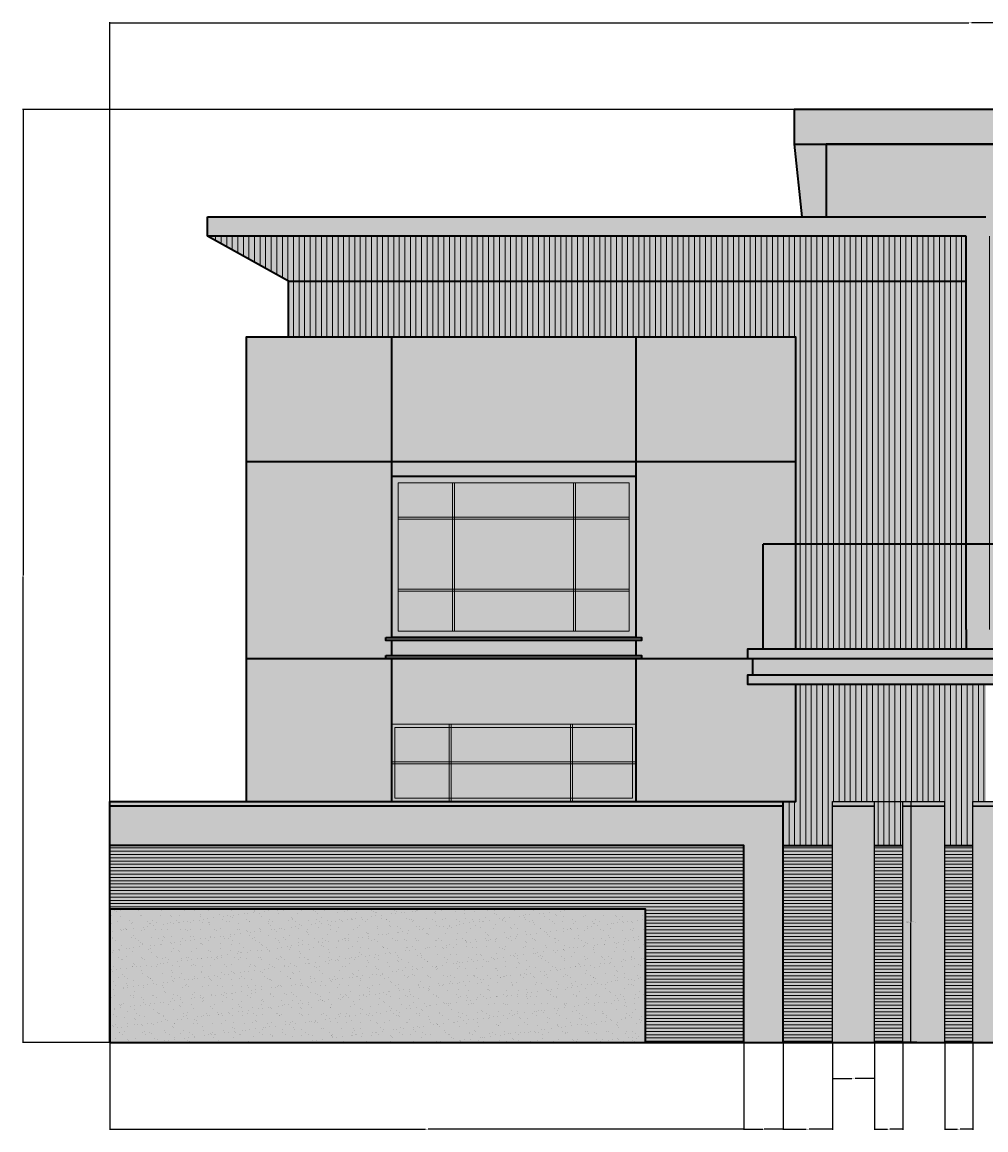
# Model space of a CAD drawing. Units: feet. Extents: x 2651 to 4047, y 949 to 1287.
# Tile 1 of 5: x 2651 to 2945, y 949 to 1287. Entities that reach past the tile are written whole.
import ezdxf

# ---------------------------------------------------------------- set-up
doc = ezdxf.new("R2010")
doc.units = ezdxf.units.FT
for name, color, linetype, lineweight in [('A-ANNO-DIMS', 2, 'Continuous', 18), ('A-ELEV', 7, 'Continuous', 35), ('A-ELEV-FNCE', 7, 'Continuous', 25), ('A-ELEV-PATT', 8, 'Continuous', 13), ('A-GLAZ', 4, 'Continuous', 18)]:
    doc.layers.add(name, color=color, linetype=linetype, lineweight=lineweight)
doc.styles.get("Standard").update_dxf_attribs({"font": 'arial.ttf'})
doc.dimstyles.get("Standard").update_dxf_attribs({"dimtxt": 0.18, "dimasz": 0.18, "dimexe": 0.18, "dimexo": 0.0625, "dimgap": 0.09, "dimtad": 0, "dimtih": 1, "dimtoh": 1, "dimdec": 1, "dimzin": 0, "dimdsep": 46, "dimlunit": 3, "dimtxsty": 'Standard', "dimcen": 0.09, "dimadec": 0, "dimazin": 0, "dimtfac": 1, "dimtdec": 1, "dimtofl": 0, "dimtmove": 0, "dimatfit": 3, "dimfxl": 1, "dimtolj": 1, "dimtzin": 0, "dimarcsym": 0})

# ---------------------------------------------------------------- blocks, each defined once
blk = doc.blocks.new('BOUNDARY-PIER-HATCHED')
for p, q in [((0, 72.1), (0, 73.54)), ((0, 72.1), (0, 73.54)), ((12.86, 0), (12.86, 73.54)), ((12.86, 0), (12.86, 73.54))]:
    blk.add_line(p, q)
for points in [[(0, 73.54), (12.86, 73.54)], [(0, 73.54), (12.86, 73.54)], [(12.86, 72.1), (0, 72.1)], [(12.86, 0), (0, 0), (0, 72.1), (12.86, 72.1)], [(12.86, 0), (0, 0), (0, 72.1), (12.86, 72.1)], [(12.86, 72.1), (0, 72.1)]]:
    blk.add_lwpolyline(points)
blk = doc.blocks.new('*D3')
at = {"layer": 'A-ANNO-DIMS', "color": 0, "lineweight": -2, "transparency": 16777216}
for p, q in [((2911.09, 1049.19), (2922.24, 1049.19)), ((2922.06, 1049.01), (2922.06, 1012.6)), ((2922.06, 975.83), (2922.06, 1012.23)), ((2911.09, 975.65), (2922.24, 975.65))]:
    blk.add_line(p, q, dxfattribs=at)
at = {"layer": 'A-ANNO-DIMS', "color": 0, "transparency": 16777216}
for points in [[(2922.03, 1049.01), (2922.09, 1049.01), (2922.06, 1049.19)], [(2922.03, 975.83), (2922.09, 975.83), (2922.06, 975.65)]]:
    blk.add_solid(points, dxfattribs=at)
at = {"layer": 'Defpoints', "color": 0, "transparency": 16777216}
for p in [(2911.03, 1049.19), (2922.06, 1049.19), (2911.03, 975.65)]:
    blk.add_point(p, dxfattribs=at)
at = {"layer": 'A-ANNO-DIMS', "color": 0, "transparency": 16777216, "insert": (2922.06, 1012.42), "char_height": 0.18, "attachment_point": 5}
blk.add_mtext('\\A1;BOUNDARY PIER 74 TYP.', dxfattribs=at)
blk = doc.blocks.new('*D4')
at = {"layer": 'A-ANNO-DIMS', "color": 0, "lineweight": -2, "transparency": 16777216}
for p, q in [((2898.17, 975.59), (2898.17, 964.44)), ((2911.03, 975.59), (2911.03, 964.44)), ((2898.35, 964.62), (2904.08, 964.62)), ((2910.85, 964.62), (2905.12, 964.62))]:
    blk.add_line(p, q, dxfattribs=at)
at = {"layer": 'A-ANNO-DIMS', "color": 0, "transparency": 16777216}
for points in [[(2898.35, 964.65), (2898.35, 964.59), (2898.17, 964.62)], [(2910.85, 964.65), (2910.85, 964.59), (2911.03, 964.62)]]:
    blk.add_solid(points, dxfattribs=at)
at = {"layer": 'Defpoints', "color": 0, "transparency": 16777216}
for p in [(2898.17, 975.65), (2911.03, 975.65), (2911.03, 964.62)]:
    blk.add_point(p, dxfattribs=at)
at = {"layer": 'A-ANNO-DIMS', "color": 0, "transparency": 16777216, "insert": (2904.6, 964.62), "char_height": 0.18, "attachment_point": 5}
blk.add_mtext('\\A1;13 TYP.', dxfattribs=at)
blk = doc.blocks.new('*D7')
at = {"layer": 'A-ANNO-DIMS', "color": 0, "lineweight": -2, "transparency": 16777216}
for p, q in [((2677.56, 975.71), (2677.56, 1287.01)), ((2677.74, 1286.83), (2939.77, 1286.83)), ((3202.59, 1286.83), (2940.56, 1286.83)), ((3202.77, 1095.71), (3202.77, 1287.01))]:
    blk.add_line(p, q, dxfattribs=at)
at = {"layer": 'A-ANNO-DIMS', "color": 0, "transparency": 16777216}
for points in [[(2677.74, 1286.86), (2677.74, 1286.8), (2677.56, 1286.83)], [(3202.59, 1286.86), (3202.59, 1286.8), (3202.77, 1286.83)]]:
    blk.add_solid(points, dxfattribs=at)
at = {"layer": 'Defpoints', "color": 0, "transparency": 16777216}
for p in [(3202.77, 1286.83), (3202.77, 1095.65), (2677.56, 975.65)]:
    blk.add_point(p, dxfattribs=at)
at = {"layer": 'A-ANNO-DIMS', "color": 0, "transparency": 16777216, "insert": (2940.17, 1286.83), "char_height": 0.18, "attachment_point": 5}
blk.add_mtext('\\A1;525.2', dxfattribs=at)
blk = doc.blocks.new('*D8')
at = {"layer": 'A-ANNO-DIMS', "color": 0, "lineweight": -2, "transparency": 16777216}
for p, q in [((3098.48, 1260.33), (2650.88, 1260.33)), ((2651.06, 1260.15), (2651.06, 1118.17)), ((2651.06, 975.83), (2651.06, 1117.81)), ((2677.49, 975.65), (2650.88, 975.65))]:
    blk.add_line(p, q, dxfattribs=at)
at = {"layer": 'A-ANNO-DIMS', "color": 0, "transparency": 16777216}
for points in [[(2651.03, 1260.15), (2651.09, 1260.15), (2651.06, 1260.33)], [(2651.03, 975.83), (2651.09, 975.83), (2651.06, 975.65)]]:
    blk.add_solid(points, dxfattribs=at)
at = {"layer": 'Defpoints', "color": 0, "transparency": 16777216}
for p in [(2651.06, 1260.33), (3098.55, 1260.33), (2677.56, 975.65)]:
    blk.add_point(p, dxfattribs=at)
at = {"layer": 'A-ANNO-DIMS', "color": 0, "transparency": 16777216, "insert": (2651.06, 1117.99), "char_height": 0.18, "attachment_point": 5}
blk.add_mtext('\\A1;284.7', dxfattribs=at)
blk = doc.blocks.new('*D9')
at = {"layer": 'A-ANNO-DIMS', "color": 0, "lineweight": -2, "transparency": 16777216}
for p, q in [((2677.56, 975.59), (2677.56, 948.97)), ((2871.06, 975.59), (2871.06, 948.97)), ((2677.74, 949.15), (2773.92, 949.15)), ((2870.88, 949.15), (2774.7, 949.15))]:
    blk.add_line(p, q, dxfattribs=at)
at = {"layer": 'A-ANNO-DIMS', "color": 0, "transparency": 16777216}
for points in [[(2677.74, 949.18), (2677.74, 949.12), (2677.56, 949.15)], [(2870.88, 949.18), (2870.88, 949.12), (2871.06, 949.15)]]:
    blk.add_solid(points, dxfattribs=at)
at = {"layer": 'Defpoints', "color": 0, "transparency": 16777216}
for p in [(2677.56, 975.65), (2871.06, 975.65), (2871.06, 949.15)]:
    blk.add_point(p, dxfattribs=at)
at = {"layer": 'A-ANNO-DIMS', "color": 0, "transparency": 16777216, "insert": (2774.31, 949.15), "char_height": 0.18, "attachment_point": 5}
blk.add_mtext('\\A1;193.5', dxfattribs=at)
blk = doc.blocks.new('*D10')
at = {"layer": 'A-ANNO-DIMS', "color": 0, "lineweight": -2, "transparency": 16777216}
for p, q in [((2871.06, 975.59), (2871.06, 948.97)), ((2883.06, 975.59), (2883.06, 948.97)), ((2871.24, 949.15), (2876.85, 949.15)), ((2882.88, 949.15), (2877.27, 949.15))]:
    blk.add_line(p, q, dxfattribs=at)
at = {"layer": 'A-ANNO-DIMS', "color": 0, "transparency": 16777216}
for points in [[(2871.24, 949.18), (2871.24, 949.12), (2871.06, 949.15)], [(2882.88, 949.18), (2882.88, 949.12), (2883.06, 949.15)]]:
    blk.add_solid(points, dxfattribs=at)
at = {"layer": 'Defpoints', "color": 0, "transparency": 16777216}
for p in [(2871.06, 975.65), (2883.06, 975.65), (2883.06, 949.15)]:
    blk.add_point(p, dxfattribs=at)
at = {"layer": 'A-ANNO-DIMS', "color": 0, "transparency": 16777216, "insert": (2877.06, 949.15), "char_height": 0.18, "attachment_point": 5}
blk.add_mtext('\\A1;12', dxfattribs=at)
blk = doc.blocks.new('*D11')
at = {"layer": 'A-ANNO-DIMS', "color": 0, "lineweight": -2, "transparency": 16777216}
for p, q in [((2883.06, 975.59), (2883.06, 948.97)), ((2898.17, 975.59), (2898.17, 948.97)), ((2883.24, 949.15), (2890.16, 949.15)), ((2897.99, 949.15), (2891.07, 949.15))]:
    blk.add_line(p, q, dxfattribs=at)
at = {"layer": 'A-ANNO-DIMS', "color": 0, "transparency": 16777216}
for points in [[(2883.24, 949.18), (2883.24, 949.12), (2883.06, 949.15)], [(2897.99, 949.18), (2897.99, 949.12), (2898.17, 949.15)]]:
    blk.add_solid(points, dxfattribs=at)
at = {"layer": 'Defpoints', "color": 0, "transparency": 16777216}
for p in [(2883.06, 975.65), (2898.17, 975.65), (2898.17, 949.15)]:
    blk.add_point(p, dxfattribs=at)
at = {"layer": 'A-ANNO-DIMS', "color": 0, "transparency": 16777216, "insert": (2890.62, 949.15), "char_height": 0.18, "attachment_point": 5}
blk.add_mtext('\\A1;15.107', dxfattribs=at)
blk = doc.blocks.new('*D12')
at = {"layer": 'A-ANNO-DIMS', "color": 0, "lineweight": -2, "transparency": 16777216}
for p, q in [((2911.03, 975.59), (2911.03, 948.97)), ((2919.6, 975.59), (2919.6, 948.97)), ((2911.21, 949.15), (2914.92, 949.15)), ((2919.42, 949.15), (2915.71, 949.15))]:
    blk.add_line(p, q, dxfattribs=at)
at = {"layer": 'A-ANNO-DIMS', "color": 0, "transparency": 16777216}
for points in [[(2911.21, 949.18), (2911.21, 949.12), (2911.03, 949.15)], [(2919.42, 949.18), (2919.42, 949.12), (2919.6, 949.15)]]:
    blk.add_solid(points, dxfattribs=at)
at = {"layer": 'Defpoints', "color": 0, "transparency": 16777216}
for p in [(2911.03, 975.65), (2919.6, 975.65), (2919.6, 949.15)]:
    blk.add_point(p, dxfattribs=at)
at = {"layer": 'A-ANNO-DIMS', "color": 0, "transparency": 16777216, "insert": (2915.31, 949.15), "char_height": 0.18, "attachment_point": 5}
blk.add_mtext('\\A1;8.576', dxfattribs=at)
blk = doc.blocks.new('*D13')
at = {"layer": 'A-ANNO-DIMS', "color": 0, "lineweight": -2, "transparency": 16777216}
for p, q in [((2932.46, 975.59), (2932.46, 948.97)), ((2941.03, 975.59), (2941.03, 948.97)), ((2932.64, 949.15), (2936.35, 949.15)), ((2940.85, 949.15), (2937.14, 949.15))]:
    blk.add_line(p, q, dxfattribs=at)
at = {"layer": 'A-ANNO-DIMS', "color": 0, "transparency": 16777216}
for points in [[(2932.64, 949.18), (2932.64, 949.12), (2932.46, 949.15)], [(2940.85, 949.18), (2940.85, 949.12), (2941.03, 949.15)]]:
    blk.add_solid(points, dxfattribs=at)
at = {"layer": 'Defpoints', "color": 0, "transparency": 16777216}
for p in [(2932.46, 975.65), (2941.03, 975.65), (2941.03, 949.15)]:
    blk.add_point(p, dxfattribs=at)
at = {"layer": 'A-ANNO-DIMS', "color": 0, "transparency": 16777216, "insert": (2936.75, 949.15), "char_height": 0.18, "attachment_point": 5}
blk.add_mtext('\\A1;8.576', dxfattribs=at)

msp = doc.modelspace()

# ---------------------------------------------------------------- hatches: boundary and pattern name
at = {"layer": 'A-ELEV-PATT'}
msp.add_hatch(color=256, dxfattribs=at).paths.add_polyline_path([(3098.5452, 1260.331), (2886.4328, 1260.331), (2886.4328, 1249.7387), (3098.5452, 1249.7387)])
h = msp.add_hatch(color=256, dxfattribs=at)
h.set_gradient(color1=(99, 100, 102), color2=(199, 200, 202), name='HEMISPHERICAL')
h.paths.add_polyline_path([(2896.1919, 1249.7387), (2886.4328, 1249.7387), (2888.7728, 1227.65), (2896.1919, 1227.65)])
h = msp.add_hatch(color=256, dxfattribs=at)
h.dxf.hatch_style = 1
h.set_gradient(color1=(199, 200, 202), tint=1, name='HEMISPHERICAL')
h.paths.add_polyline_path([(3169.7582, 1242.6921), (3109.1174, 1227.65), (3169.7582, 1227.65)])
h.paths.add_polyline_path([(3088.7861, 1249.7387), (2896.1919, 1249.7387), (2896.1919, 1227.65), (2944.9934, 1227.65), (2944.9934, 1221.65), (2962.7341, 1221.65), (2962.7341, 1238.6943), (3088.7861, 1238.6943)])
h = msp.add_hatch(color=256, dxfattribs=at)
h.dxf.hatch_style = 1
h.paths.add_polyline_path([(2944.9934, 1227.65), (2896.1919, 1227.65), (2707.3507, 1227.65), (2707.3507, 1221.65), (2938.9934, 1221.65), (2938.9934, 1127.711), (2944.9934, 1127.711), (2944.9934, 1221.65)])
h.paths.add_polyline_path([(2944.9934, 1127.711), (2938.9934, 1127.711), (2938.9934, 1101.65), (2938.9934, 1095.65), (3196.0086, 1095.65), (3196.0086, 1101.65), (3180.6945, 1101.65), (3180.6945, 1127.711), (3169.7582, 1127.711), (3169.7582, 1101.65), (3097.3565, 1101.65), (3002.0224, 1101.65), (2944.9934, 1101.65)])
h.paths.add_polyline_path([(3180.6945, 1242.6921), (3169.7582, 1242.6921), (3169.7582, 1221.65), (3169.7582, 1127.711), (3180.6945, 1127.711)])
h = msp.add_hatch(color=256, dxfattribs=at)
h.set_gradient(color1=(199, 200, 202), color2=(199, 200, 202), tint=1, name='HEMISPHERICAL')
h.paths.add_polyline_path([(2763.5286, 1190.8721), (2719.1033, 1190.8721), (2719.1033, 1152.9072), (2763.5286, 1152.9072)])
h.paths.add_polyline_path([(2838.0977, 1190.8721), (2763.5286, 1190.8721), (2763.5286, 1152.9072), (2838.0977, 1152.9072)])
h.paths.add_polyline_path([(2887.0237, 1190.8721), (2838.0977, 1190.8721), (2838.0977, 1152.9072), (2887.0237, 1152.9072)])
h.paths.add_polyline_path([(2877.0224, 1127.711), (2887.0237, 1127.711), (2887.0237, 1152.9072), (2838.0977, 1152.9072), (2838.0977, 1099.175), (2839.8136, 1099.175), (2839.8136, 1098.3392), (2838.0977, 1098.3392), (2838.0977, 1093.6891), (2839.8136, 1093.6891), (2839.8136, 1092.8533), (2872.1973, 1092.8533), (2872.1973, 1095.65), (2877.0224, 1095.65)])
h.paths.add_polyline_path([(2887.0237, 1127.711), (2877.0224, 1127.711), (2877.0224, 1095.65), (2887.0237, 1095.65)], flags=17)
h.paths.add_polyline_path([(2887.0237, 1084.9772), (2872.1973, 1084.9772), (2872.1973, 1087.7738), (2873.8204, 1087.7738), (2873.8204, 1092.8533), (2872.1973, 1092.8533), (2838.0977, 1092.8533), (2838.0977, 1049.1862), (2887.0237, 1049.1862)])
h.paths.add_polyline_path([(2763.5286, 1152.9072), (2719.1033, 1152.9072), (2719.1033, 1092.8533), (2761.8127, 1092.8533), (2761.8127, 1093.6891), (2763.5286, 1093.6891), (2763.5286, 1098.3392), (2761.8127, 1098.3392), (2761.8127, 1099.175), (2763.5286, 1099.175)])
h.paths.add_polyline_path([(2763.5286, 1092.8533), (2719.1033, 1092.8533), (2719.1033, 1049.1862), (2763.5286, 1049.1862), (2763.5286, 1072.7574)])
h.paths.add_polyline_path([(2838.0977, 1152.9072), (2763.5286, 1152.9072), (2763.5286, 1148.4143), (2838.0977, 1148.4143)])
h.paths.add_polyline_path([(2838.0977, 1092.8533), (2763.5286, 1092.8533), (2763.5286, 1072.7574), (2838.0977, 1072.7574)])
h.paths.add_polyline_path([(2883.0637, 1047.7503), (2677.5561, 1047.7503), (2677.5561, 1035.7503), (2871.0637, 1035.7503), (2871.0637, 975.65), (2883.0637, 975.65)])
h.paths.add_polyline_path([(2911.0266, 1047.7503), (2898.171, 1047.7503), (2898.171, 975.65), (2911.0266, 975.65)])
h.paths.add_polyline_path([(2932.4585, 1047.7503), (2919.6029, 1047.7503), (2919.6029, 975.65), (2932.4585, 975.65)])
h.paths.add_polyline_path([(2953.8904, 1047.7503), (2941.0349, 1047.7503), (2941.0349, 975.65), (2953.8904, 975.65)])
h.paths.add_polyline_path([(2985.9915, 1047.7503), (2962.4668, 1047.7503), (2962.4668, 975.65), (2975.3223, 975.65), (2985.9915, 975.65)])
h.paths.add_polyline_path([(3097.3565, 1221.65), (3097.3565, 1238.6943), (3054.2372, 1238.6943), (3054.2372, 1163.1131), (3097.3565, 1163.1131)])
h.paths.add_polyline_path([(3002.0224, 1238.6943), (2962.7341, 1238.6943), (2962.7341, 1163.1131), (3002.0224, 1163.1131)])
h.paths.add_polyline_path([(3054.2372, 1238.6943), (3002.0224, 1238.6943), (3002.0224, 1163.1131), (3054.2372, 1163.1131)])
h.paths.add_polyline_path([(3002.0224, 1163.1131), (2962.7341, 1163.1131), (2962.7341, 1127.711), (3002.0224, 1127.711)])
h.paths.add_polyline_path([(3002.0224, 1127.711), (2962.7341, 1127.711), (2962.7341, 1101.65), (3002.0224, 1101.65)])
h.paths.add_polyline_path([(3097.3565, 1163.1131), (3054.2372, 1163.1131), (3054.2372, 1127.711), (3097.3565, 1127.711)])
h.paths.add_polyline_path([(3097.3565, 1127.711), (3054.2372, 1127.711), (3054.2372, 1101.65), (3097.3565, 1101.65)])
h = msp.add_hatch(color=256, dxfattribs=at)
h.set_gradient(color1=(168, 95, 18), color2=(168, 95, 18), tint=1, name='CURVED')
h.paths.add_polyline_path([(2938.9934, 1207.954), (2732.0644, 1207.954), (2732.0644, 1190.8721), (2887.0237, 1190.8721), (2887.0237, 1127.711), (2938.9934, 1127.711)])
h.paths.add_polyline_path([(2938.9934, 1221.65), (2707.3507, 1221.65), (2732.0644, 1207.954), (2938.9934, 1207.954)])
h.paths.add_polyline_path([(3169.7582, 1221.65), (3097.3565, 1221.65), (3097.3565, 1127.711), (3169.7582, 1127.711)])
h.paths.add_polyline_path([(2962.7341, 1221.65), (2944.9934, 1221.65), (2944.9934, 1127.711), (2962.7341, 1127.711)])
h.paths.add_polyline_path([(3169.7582, 1227.65), (3097.3565, 1227.65), (3097.3565, 1221.65), (3169.7582, 1221.65)])
h.paths.add_polyline_path([(3169.7582, 1127.711), (3097.3565, 1127.711), (3097.3565, 1101.65), (3169.7582, 1101.65)])
h.paths.add_polyline_path([(2962.7341, 1127.711), (2944.9934, 1127.711), (2944.9934, 1101.65), (2962.7341, 1101.65)])
h.paths.add_polyline_path([(2938.9934, 1127.711), (2887.0237, 1127.711), (2887.0237, 1095.65), (2938.9934, 1095.65), (2938.9934, 1101.65)])
h.paths.add_polyline_path([(2944.9934, 1084.9772), (2887.0237, 1084.9772), (2887.0237, 1049.1862), (2883.0637, 1049.1862), (2883.0637, 1047.7503), (2883.0637, 1035.7503), (2898.171, 1035.7503), (2898.171, 1047.7503), (2898.171, 1049.1862), (2911.0266, 1049.1862), (2911.0266, 1035.7503), (2919.6029, 1035.7503), (2919.6029, 1047.7503), (2919.6029, 1049.1862), (2932.4585, 1049.1862), (2932.4585, 1035.7503), (2941.0349, 1035.7503), (2941.0349, 1047.7503), (2941.0349, 1049.1862), (2944.9934, 1049.1862)])
h = msp.add_hatch(dxfattribs=at)
h.set_pattern_fill('_USER', color=256, scale=1.7, angle=90, style=0, pattern_type=0)
h.set_pattern_definition([(90, (0, 0), (-1.7, 1e-16), [])])
h.paths.add_polyline_path([(2938.9934, 1207.954), (2732.0644, 1207.954), (2732.0644, 1190.8721), (2887.0237, 1190.8721), (2887.0237, 1127.711), (2938.9934, 1127.711)])
h.paths.add_polyline_path([(2938.9934, 1221.65), (2707.3507, 1221.65), (2732.0644, 1207.954), (2938.9934, 1207.954)])
h.paths.add_polyline_path([(2938.9934, 1127.711), (2887.0237, 1127.711), (2887.0237, 1095.65), (2938.9934, 1095.65), (2938.9934, 1101.65)])
h.paths.add_polyline_path([(2962.7341, 1221.65), (2944.9934, 1221.65), (2944.9934, 1127.711), (2962.7341, 1127.711)])
h.paths.add_polyline_path([(2962.7341, 1127.711), (2944.9934, 1127.711), (2944.9934, 1101.65), (2962.7341, 1101.65)])
h.paths.add_polyline_path([(3169.7582, 1221.65), (3097.3565, 1221.65), (3097.3565, 1127.711), (3169.7582, 1127.711)])
h.paths.add_polyline_path([(3169.7582, 1227.65), (3097.3565, 1227.65), (3097.3565, 1221.65), (3169.7582, 1221.65)])
h.paths.add_polyline_path([(3169.7582, 1127.711), (3097.3565, 1127.711), (3097.3565, 1101.65), (3169.7582, 1101.65)])
h.paths.add_polyline_path([(2944.9934, 1084.9772), (2887.0237, 1084.9772), (2887.0237, 1049.1862), (2883.0637, 1049.1862), (2883.0637, 1047.7503), (2883.0637, 1035.7503), (2898.171, 1035.7503), (2898.171, 1047.7503), (2898.171, 1049.1862), (2911.0266, 1049.1862), (2911.0266, 1035.7503), (2919.6029, 1035.7503), (2919.6029, 1047.7503), (2919.6029, 1049.1862), (2932.4585, 1049.1862), (2932.4585, 1035.7503), (2941.0349, 1035.7503), (2941.0349, 1047.7503), (2941.0349, 1049.1862), (2944.9934, 1049.1862)])
h = msp.add_hatch(dxfattribs=at)
h.set_pattern_fill('AR-SAND', color=256, scale=0.09, style=0)
h.set_pattern_definition([(37.5, (-817.72, 3e-12), (-0.1440028, 4.404719), [0, -3.47472, 0, -3.8862, 0, -3.71475]), (7.5, (-817.72, 3e-12), (4.0457095, 6.451426), [0, -1.87452, 0, -3.13182, 0, -1.20015]), (327.5, (-820.5318, 3e-12), (7.1189313, 0.0129347), [0, -1.143, 0, -4.1148, 0, -5.3721]), (317.5, (-820.532, 3e-12), (6.872008, 2.006364), [0, -0.5715, 0, -2.69748, 0, -3.0861])])
h.paths.add_polyline_path([(2763.5286, 1190.8721), (2719.1033, 1190.8721), (2719.1033, 1152.9072), (2763.5286, 1152.9072)])
h.paths.add_polyline_path([(2838.0977, 1190.8721), (2763.5286, 1190.8721), (2763.5286, 1152.9072), (2838.0977, 1152.9072)])
h.paths.add_polyline_path([(2887.0237, 1190.8721), (2838.0977, 1190.8721), (2838.0977, 1152.9072), (2887.0237, 1152.9072)])
h.paths.add_polyline_path([(2838.0977, 1152.9072), (2763.5286, 1152.9072), (2763.5286, 1148.4143), (2838.0977, 1148.4143)])
h.paths.add_polyline_path([(2887.0237, 1152.9072), (2838.0977, 1152.9072), (2838.0977, 1099.175), (2839.8136, 1099.175), (2839.8136, 1098.3392), (2838.0977, 1098.3392), (2838.0977, 1093.6891), (2839.8136, 1093.6891), (2839.8136, 1092.8533), (2872.1973, 1092.8533), (2872.1973, 1095.65), (2877.0224, 1095.65), (2877.0224, 1127.711), (2887.0237, 1127.711)])
h.paths.add_polyline_path([(2887.0237, 1127.711), (2877.0224, 1127.711), (2877.0224, 1095.65), (2887.0237, 1095.65)], flags=17)
h.paths.add_polyline_path([(2763.5286, 1152.9072), (2719.1033, 1152.9072), (2719.1033, 1092.8533), (2761.8127, 1092.8533), (2761.8127, 1093.6891), (2763.5286, 1093.6891), (2763.5286, 1098.3392), (2761.8127, 1098.3392), (2761.8127, 1099.175), (2763.5286, 1099.175)])
h.paths.add_polyline_path([(2763.5286, 1092.8533), (2761.8127, 1092.8533), (2719.1033, 1092.8533), (2719.1033, 1049.1862), (2763.5286, 1049.1862)])
h.paths.add_polyline_path([(2887.0237, 1084.9772), (2872.1973, 1084.9772), (2872.1973, 1087.7738), (2873.8204, 1087.7738), (2873.8204, 1092.8533), (2872.1973, 1092.8533), (2838.0977, 1092.8533), (2838.0977, 1049.1862), (2887.0237, 1049.1862)])
h.paths.add_polyline_path([(2838.0977, 1092.8533), (2763.5286, 1092.8533), (2763.5286, 1072.7574), (2838.0977, 1072.7574)])
h.paths.add_polyline_path([(2911.0266, 1047.7503), (2898.171, 1047.7503), (2898.171, 975.65), (2911.0266, 975.65)])
h.paths.add_polyline_path([(2932.4585, 1047.7503), (2919.6029, 1047.7503), (2919.6029, 975.65), (2932.4585, 975.65)])
h.paths.add_polyline_path([(2953.8904, 1047.7503), (2941.0349, 1047.7503), (2941.0349, 975.65), (2953.8904, 975.65)])
h.paths.add_polyline_path([(2985.9915, 1047.7503), (2962.4668, 1047.7503), (2962.4668, 975.65), (2975.3223, 975.65), (2985.9915, 975.65)])
h.paths.add_polyline_path([(2883.0637, 1047.7503), (2677.5561, 1047.7503), (2677.5561, 1035.7503), (2871.0637, 1035.7503), (2871.0637, 975.65), (2883.0637, 975.65)])
h = msp.add_hatch(color=256, dxfattribs=at)
h.paths.add_polyline_path([(2838.0977, 1148.4143), (2763.5286, 1148.4143), (2763.5286, 1099.175), (2838.0977, 1099.175)])
h.paths.add_polyline_path([(2836.0977, 1146.4143), (2836.0977, 1101.175), (2765.5286, 1101.175), (2765.5286, 1146.4143)], flags=16)
h.paths.add_polyline_path([(2819.7437, 1135.9058), (2819.7437, 1113.3773), (2782.111, 1113.3773), (2782.111, 1135.9058)], flags=0)
h.paths.add_polyline_path([(2819.1363, 1135.3515), (2819.1363, 1113.9316), (2782.7185, 1113.9316), (2782.7185, 1135.3515)], flags=0)
h.paths.add_polyline_path([(2782.7185, 1146.4143), (2782.111, 1146.4143), (2782.111, 1135.9058), (2782.7185, 1135.9058)], flags=0)
h.paths.add_polyline_path([(2782.111, 1135.9058), (2765.5286, 1135.9058), (2765.5286, 1135.3515), (2782.111, 1135.3515)], flags=0)
h.paths.add_polyline_path([(2836.0977, 1135.9058), (2819.7437, 1135.9058), (2819.7437, 1135.3515), (2836.0977, 1135.3515)], flags=0)
h.paths.add_polyline_path([(2819.7437, 1146.4143), (2819.1363, 1146.4143), (2819.1363, 1135.9058), (2819.7437, 1135.9058)], flags=0)
h.paths.add_polyline_path([(2836.0977, 1113.9316), (2819.7437, 1113.9316), (2819.7437, 1113.3773), (2836.0977, 1113.3773)], flags=0)
h.paths.add_polyline_path([(2819.7437, 1113.3773), (2819.1363, 1113.3773), (2819.1363, 1101.175), (2819.7437, 1101.175)], flags=0)
h.paths.add_polyline_path([(2782.111, 1113.9316), (2765.5286, 1113.9316), (2765.5286, 1113.3773), (2782.111, 1113.3773)], flags=0)
h.paths.add_polyline_path([(2782.7185, 1113.3773), (2782.111, 1113.3773), (2782.111, 1101.175), (2782.7185, 1101.175)], flags=0)
h.paths.add_polyline_path([(2781.7185, 1061.2489), (2781.111, 1061.2489), (2781.111, 1060.6946), (2781.7185, 1060.6946)])
h.paths.add_polyline_path([(2781.7185, 1072.7574), (2781.111, 1072.7574), (2781.111, 1061.2489), (2781.7185, 1061.2489)])
h.paths.add_polyline_path([(2838.0977, 1061.2489), (2781.7185, 1061.2489), (2781.7185, 1060.6946), (2838.0977, 1060.6946)])
h.paths.add_polyline_path([(2781.111, 1061.2489), (2763.5286, 1061.2489), (2763.5286, 1060.6946), (2781.111, 1060.6946)])
h.paths.add_polyline_path([(2781.7185, 1060.6946), (2781.111, 1060.6946), (2781.111, 1049.1862), (2781.7185, 1049.1862)])
h.paths.add_polyline_path([(2781.111, 1072.7574), (2763.5286, 1072.7574), (2763.5286, 1061.2489), (2764.5286, 1061.2489), (2764.5286, 1071.7574), (2781.111, 1071.7574)])
h.paths.add_polyline_path([(2838.0977, 1072.7574), (2781.7185, 1072.7574), (2781.7185, 1071.7574), (2837.0977, 1071.7574), (2837.0977, 1061.2489), (2838.0977, 1061.2489)])
h.paths.add_polyline_path([(2838.0977, 1060.6946), (2837.0977, 1060.6946), (2837.0977, 1050.1862), (2781.7185, 1050.1862), (2781.7185, 1049.1862), (2838.0977, 1049.1862)])
h.paths.add_polyline_path([(2764.5286, 1060.6946), (2763.5286, 1060.6946), (2763.5286, 1049.1862), (2781.111, 1049.1862), (2781.111, 1050.1862), (2764.5286, 1050.1862)])
h.paths.add_polyline_path([(2818.7437, 1071.7574), (2818.1363, 1071.7574), (2818.1363, 1061.2489), (2818.7437, 1061.2489)], flags=17)
h.paths.add_polyline_path([(2818.7437, 1060.6946), (2818.1363, 1060.6946), (2818.1363, 1050.1862), (2818.7437, 1050.1862)], flags=17)
h.paths.add_polyline_path([(2883.0637, 1049.1862), (2719.1033, 1049.1862), (2677.5561, 1049.1862), (2677.5561, 1047.7503), (2883.0637, 1047.7503)])
h.paths.add_polyline_path([(2911.0266, 1049.1862), (2898.171, 1049.1862), (2898.171, 1047.7503), (2911.0266, 1047.7503)])
h.paths.add_polyline_path([(2932.4585, 1049.1862), (2919.6029, 1049.1862), (2919.6029, 1047.7503), (2932.4585, 1047.7503)])
h.paths.add_polyline_path([(2953.8904, 1049.1862), (2941.0349, 1049.1862), (2941.0349, 1047.7503), (2953.8904, 1047.7503)])
h.paths.add_polyline_path([(2985.9915, 1049.1862), (2962.4668, 1049.1862), (2962.4668, 1047.7503), (2985.9915, 1047.7503)])
h.paths.add_polyline_path([(3007.2777, 1077.1763), (2981.6074, 1077.1763), (2981.6074, 1049.1862), (2982.6074, 1049.1862), (2982.6074, 1076.1763), (3006.2777, 1076.1763), (3006.2777, 1038.5677), (2985.9915, 1038.5677), (2985.9915, 1037.5677), (3007.2777, 1037.5677)])
h.paths.add_polyline_path([(3060.9744, 1069.9768), (3047.3083, 1069.9768), (3047.3083, 1058.6821), (3060.9744, 1058.6821)])
h.paths.add_polyline_path([(3059.9744, 1068.9768), (3059.9744, 1059.6821), (3048.3083, 1059.6821), (3048.3083, 1068.9768)], flags=16)
h = msp.add_hatch(color=256, dxfattribs=at)
h.set_gradient(color1=(194, 211, 228), color2=(194, 211, 228), name='HEMISPHERICAL')
h.paths.add_polyline_path([(2819.1363, 1135.3515), (2782.7185, 1135.3515), (2782.7185, 1113.9316), (2819.1363, 1113.9316)])
h.paths.add_polyline_path([(2782.111, 1146.4143), (2765.5286, 1146.4143), (2765.5286, 1135.9058), (2782.111, 1135.9058)])
h.paths.add_polyline_path([(2819.1363, 1146.4143), (2782.7185, 1146.4143), (2782.7185, 1135.9058), (2819.1363, 1135.9058)])
h.paths.add_polyline_path([(2782.111, 1135.3515), (2765.5286, 1135.3515), (2765.5286, 1113.9316), (2782.111, 1113.9316)])
h.paths.add_polyline_path([(2836.0977, 1146.4143), (2819.7437, 1146.4143), (2819.7437, 1135.9058), (2836.0977, 1135.9058)])
h.paths.add_polyline_path([(2836.0977, 1135.3515), (2819.7437, 1135.3515), (2819.7437, 1113.9316), (2836.0977, 1113.9316)])
h.paths.add_polyline_path([(2836.0977, 1113.3773), (2819.7437, 1113.3773), (2819.7437, 1101.175), (2836.0977, 1101.175)])
h.paths.add_polyline_path([(2819.1363, 1113.3773), (2782.7185, 1113.3773), (2782.7185, 1101.175), (2819.1363, 1101.175)])
h.paths.add_polyline_path([(2782.111, 1113.3773), (2765.5286, 1113.3773), (2765.5286, 1101.175), (2782.111, 1101.175)])
h.paths.add_polyline_path([(2781.111, 1060.6946), (2764.5286, 1060.6946), (2764.5286, 1050.1862), (2781.111, 1050.1862)])
h.paths.add_polyline_path([(2818.1363, 1060.6946), (2781.7185, 1060.6946), (2781.7185, 1050.1862), (2818.1363, 1050.1862)])
h.paths.add_polyline_path([(2837.0977, 1060.6946), (2818.7437, 1060.6946), (2818.7437, 1050.1862), (2837.0977, 1050.1862)])
h.paths.add_polyline_path([(2837.0977, 1071.7574), (2818.7437, 1071.7574), (2818.7437, 1061.2489), (2837.0977, 1061.2489)])
h.paths.add_polyline_path([(2818.1363, 1071.7574), (2781.7185, 1071.7574), (2781.7185, 1061.2489), (2818.1363, 1061.2489)])
h.paths.add_polyline_path([(2781.111, 1071.7574), (2764.5286, 1071.7574), (2764.5286, 1061.2489), (2781.111, 1061.2489)])
h.paths.add_polyline_path([(3006.2777, 1076.1763), (2982.6074, 1076.1763), (2982.6074, 1049.1862), (2985.9915, 1049.1862), (2985.9915, 1038.5677), (3006.2777, 1038.5677)])
h = msp.add_hatch(color=256, dxfattribs=at)
h.set_gradient(color1=(120, 68, 13), color2=(120, 68, 13), name='HEMISPHERICAL')
h.paths.add_polyline_path([(2839.8136, 1099.175), (2761.8127, 1099.175), (2761.8127, 1098.3392), (2839.8136, 1098.3392)])
h.paths.add_polyline_path([(2839.8136, 1093.6891), (2761.8127, 1093.6891), (2761.8127, 1092.8533), (2839.8136, 1092.8533)])
h.paths.add_polyline_path([(3202.774, 1095.65), (2872.1973, 1095.65), (2872.1973, 1092.8533), (3202.774, 1092.8533)])
h.paths.add_polyline_path([(3202.774, 1087.7738), (2872.1973, 1087.7738), (2872.1973, 1084.9772), (3202.774, 1084.9772)])
h = msp.add_hatch(color=256, dxfattribs=at)
h.paths.add_polyline_path([(2838.0977, 1098.3392), (2763.5286, 1098.3392), (2763.5286, 1093.6891), (2838.0977, 1093.6891)])
h.paths.add_polyline_path([(3200.884, 1092.8533), (2873.8204, 1092.8533), (2873.8204, 1087.7738), (3200.884, 1087.7738)])
h = msp.add_hatch(color=256, dxfattribs=at)
h.set_gradient(color1=(120, 68, 13), color2=(120, 68, 13), name='CURVED')
h.paths.add_polyline_path([(2871.0637, 1035.7503), (2677.5561, 1035.7503), (2677.5561, 1016.3476), (2841.0579, 1016.3476), (2841.0579, 975.65), (2871.0637, 975.65)])
h.paths.add_polyline_path([(2898.171, 1035.7503), (2883.0637, 1035.7503), (2883.0637, 975.65), (2898.171, 975.65)])
h.paths.add_polyline_path([(2919.6029, 1035.7503), (2911.0266, 1035.7503), (2911.0266, 975.65), (2919.6029, 975.65)])
h.paths.add_polyline_path([(2941.0349, 1035.7503), (2932.4585, 1035.7503), (2932.4585, 975.65), (2941.0349, 975.65)])
h.paths.add_polyline_path([(2962.4668, 1035.7503), (2953.8904, 1035.7503), (2953.8904, 975.65), (2962.4668, 975.65)])
h = msp.add_hatch(dxfattribs=at)
h.set_pattern_fill('_USER', color=256, style=0, pattern_type=0)
h.set_pattern_definition([(0, (0, 0), (0, 1), [])])
h.paths.add_polyline_path([(2871.0637, 1035.7503), (2677.5561, 1035.7503), (2677.5561, 1016.3476), (2841.0579, 1016.3476), (2841.0579, 975.65), (2871.0637, 975.65)])
h.paths.add_polyline_path([(2898.171, 1035.7503), (2883.0637, 1035.7503), (2883.0637, 975.65), (2898.171, 975.65)])
h.paths.add_polyline_path([(2919.6029, 1035.7503), (2911.0266, 1035.7503), (2911.0266, 975.65), (2919.6029, 975.65)])
h.paths.add_polyline_path([(2941.0349, 1035.7503), (2932.4585, 1035.7503), (2932.4585, 975.65), (2941.0349, 975.65)])
h.paths.add_polyline_path([(2962.4668, 1035.7503), (2953.8904, 1035.7503), (2953.8904, 975.65), (2962.4668, 975.65)])
h = msp.add_hatch(color=256, dxfattribs=at)
h.set_gradient(color1=(199, 200, 202), color2=(199, 200, 202), tint=1, name='HEMISPHERICAL')
h.paths.add_polyline_path([(2841.0579, 1016.3476), (2677.5561, 1016.3476), (2677.5561, 975.65), (2841.0579, 975.65)])
h = msp.add_hatch(dxfattribs=at)
h.set_pattern_fill('AR-SAND', color=256, scale=0.09, style=0)
h.paths.add_polyline_path([(2841.0579, 1016.3476), (2677.5561, 1016.3476), (2677.5561, 975.65), (2841.0579, 975.65)])

# ---------------------------------------------------------------- linework, layer by layer
at = {"layer": 'A-ELEV'}
for p, q in [((2886.4328, 1249.7387), (2888.7728, 1227.65)), ((2886.4328, 1249.7387), (2888.7728, 1227.65)), ((2707.3507, 1227.65), (2944.9934, 1227.65)), ((2707.3507, 1221.65), (2707.3507, 1227.65)), ((2707.3507, 1227.65), (2944.9934, 1227.65)), ((2707.3507, 1221.65), (2707.3507, 1227.65)), ((2732.0644, 1207.954), (2707.3507, 1221.65)), ((2938.9934, 1221.65), (2707.3507, 1221.65)), ((2938.9934, 1221.65), (2707.3507, 1221.65)), ((2732.0644, 1207.954), (2707.3507, 1221.65)), ((2732.0644, 1190.8721), (2732.0644, 1207.954)), ((2732.0644, 1207.954), (2938.9934, 1207.954)), ((2732.0644, 1190.8721), (2732.0644, 1207.954)), ((2732.0644, 1207.954), (2938.9934, 1207.954)), ((2763.5286, 1190.8721), (2763.5286, 1099.175)), ((2763.5286, 1190.8721), (2763.5286, 1099.175)), ((2838.0977, 1190.8721), (2838.0977, 1099.175)), ((2838.0977, 1190.8721), (2838.0977, 1099.175)), ((2719.1033, 1152.9072), (2887.0237, 1152.9072)), ((2719.1033, 1152.9072), (2887.0237, 1152.9072)), ((3196.0086, 1127.711), (2877.0224, 1127.711)), ((2877.0224, 1095.65), (2877.0224, 1127.711)), ((3196.0086, 1127.711), (2877.0224, 1127.711)), ((2877.0224, 1095.65), (2877.0224, 1127.711)), ((2938.9934, 1101.65), (2938.9934, 1095.65)), ((2938.9934, 1101.65), (2938.9934, 1095.65)), ((2763.5286, 1098.3392), (2763.5286, 1093.6891)), ((2763.5286, 1098.3392), (2763.5286, 1093.6891)), ((2838.0977, 1098.3392), (2838.0977, 1093.6891)), ((2838.0977, 1098.3392), (2838.0977, 1093.6891)), ((3196.0086, 1095.65), (2887.0237, 1095.65)), ((3196.0086, 1095.65), (2887.0237, 1095.65)), ((2719.1033, 1092.8533), (2887.0237, 1092.8533)), ((2719.1033, 1092.8533), (2887.0237, 1092.8533)), ((2763.5286, 1092.8533), (2763.5286, 1049.1862)), ((2763.5286, 1092.8533), (2763.5286, 1049.1862)), ((2838.0977, 1092.8533), (2838.0977, 1049.1862)), ((2838.0977, 1092.8533), (2838.0977, 1049.1862)), ((2677.5561, 975.65), (2677.5561, 1049.1862)), ((2677.5561, 975.65), (2677.5561, 1049.1862)), ((2883.0637, 1047.7503), (2883.0637, 1049.1862)), ((2883.0637, 1047.7503), (2883.0637, 1049.1862)), ((2883.0637, 1035.7503), (2898.171, 1035.7503)), ((2883.0637, 1035.7503), (2898.171, 1035.7503)), ((2911.0266, 1035.7503), (2919.6029, 1035.7503)), ((2911.0266, 1035.7503), (2919.6029, 1035.7503)), ((2932.4585, 1035.7503), (2941.0349, 1035.7503)), ((2932.4585, 1035.7503), (2941.0349, 1035.7503)), ((2677.5561, 975.65), (3196.0086, 975.65)), ((2677.5561, 975.65), (3196.0086, 975.65))]:
    msp.add_line(p, q, dxfattribs=at)
for points in [[(2886.4328, 1249.7387), (3098.5452, 1249.7387), (3098.5452, 1260.331), (2886.4328, 1260.331)], [(2886.4328, 1249.7387), (3098.5452, 1249.7387), (3098.5452, 1260.331), (2886.4328, 1260.331)], [(2761.8127, 1099.175), (2839.8136, 1099.175), (2839.8136, 1098.3392), (2761.8127, 1098.3392)], [(2761.8127, 1099.175), (2839.8136, 1099.175), (2839.8136, 1098.3392), (2761.8127, 1098.3392)], [(3202.774, 1095.65), (2872.1973, 1095.65), (2872.1973, 1092.8533), (3202.774, 1092.8533)], [(3202.774, 1095.65), (2872.1973, 1095.65), (2872.1973, 1092.8533), (3202.774, 1092.8533)], [(2761.8127, 1093.6891), (2839.8136, 1093.6891), (2839.8136, 1092.8533), (2761.8127, 1092.8533)], [(2761.8127, 1093.6891), (2839.8136, 1093.6891), (2839.8136, 1092.8533), (2761.8127, 1092.8533)], [(2873.8204, 1092.8533), (3200.884, 1092.8533), (3200.884, 1087.7738), (2873.8204, 1087.7738)], [(2873.8204, 1092.8533), (3200.884, 1092.8533), (3200.884, 1087.7738), (2873.8204, 1087.7738)], [(3202.774, 1087.7738), (2872.1973, 1087.7738), (2872.1973, 1084.9772), (3202.774, 1084.9772)], [(3202.774, 1087.7738), (2872.1973, 1087.7738), (2872.1973, 1084.9772), (3202.774, 1084.9772)], [(2677.5561, 975.65), (2841.0579, 975.65), (2841.0579, 1016.3476), (2677.5561, 1016.3476)]]:
    msp.add_lwpolyline(points, close=True, dxfattribs=at)
for points in [[(3088.7861, 1238.6943), (3088.7861, 1249.7387), (2896.1919, 1249.7387), (2896.1919, 1227.65), (2944.9934, 1227.65)], [(3088.7861, 1238.6943), (3088.7861, 1249.7387), (2896.1919, 1249.7387), (2896.1919, 1227.65), (2944.9934, 1227.65)], [(2938.9934, 1101.65), (2938.9934, 1221.65)], [(2938.9934, 1101.65), (2938.9934, 1221.65)], [(2887.0237, 1095.65), (2887.0237, 1190.8721), (2719.1033, 1190.8721), (2719.1033, 1049.1862), (2887.0237, 1049.1862), (2887.0237, 1084.9772)], [(2887.0237, 1095.65), (2887.0237, 1190.8721), (2719.1033, 1190.8721), (2719.1033, 1049.1862), (2887.0237, 1049.1862), (2887.0237, 1084.9772)], [(2763.5286, 1148.4143), (2838.0977, 1148.4143)], [(2763.5286, 1148.4143), (2838.0977, 1148.4143)], [(2838.0977, 1099.175), (2763.5286, 1099.175)], [(2838.0977, 1099.175), (2763.5286, 1099.175)], [(2883.0637, 1047.7503), (2677.5561, 1047.7503), (2677.5561, 1049.1862), (2883.0637, 1049.1862)], [(2883.0637, 1047.7503), (2677.5561, 1047.7503), (2677.5561, 1049.1862), (2883.0637, 1049.1862)], [(2883.0637, 975.65), (2883.0637, 1047.7503), (2677.5561, 1047.7503)], [(2883.0637, 975.65), (2883.0637, 1047.7503), (2677.5561, 1047.7503)], [(2871.0637, 975.65), (2871.0637, 1035.7503), (2677.5561, 1035.7503)], [(2871.0637, 975.65), (2871.0637, 1035.7503), (2677.5561, 1035.7503)], [(2923.8822, 975.65), (2919.6029, 975.65)], [(2923.8822, 975.65), (2919.6029, 975.65)]]:
    msp.add_lwpolyline(points, dxfattribs=at)
at = {"layer": 'A-GLAZ'}
for points in [[(2765.5286, 1146.4143), (2836.0977, 1146.4143), (2836.0977, 1101.175), (2765.5286, 1101.175)], [(2765.5286, 1146.4143), (2836.0977, 1146.4143), (2836.0977, 1101.175), (2765.5286, 1101.175)], [(2838.0977, 1049.1862), (2763.5286, 1049.1862), (2763.5286, 1072.7574), (2838.0977, 1072.7574)], [(2838.0977, 1049.1862), (2763.5286, 1049.1862), (2763.5286, 1072.7574), (2838.0977, 1072.7574)], [(2837.0977, 1050.1862), (2764.5286, 1050.1862), (2764.5286, 1071.7574), (2837.0977, 1071.7574)], [(2837.0977, 1050.1862), (2764.5286, 1050.1862), (2764.5286, 1071.7574), (2837.0977, 1071.7574)], [(2781.111, 1072.7574), (2781.7185, 1072.7574), (2781.7185, 1049.1862), (2781.111, 1049.1862)], [(2781.111, 1072.7574), (2781.7185, 1072.7574), (2781.7185, 1049.1862), (2781.111, 1049.1862)], [(2818.1363, 1072.7574), (2818.7437, 1072.7574), (2818.7437, 1049.1862), (2818.1363, 1049.1862)], [(2818.1363, 1072.7574), (2818.7437, 1072.7574), (2818.7437, 1049.1862), (2818.1363, 1049.1862)], [(2763.5286, 1061.2489), (2838.0977, 1061.2489), (2838.0977, 1060.6946), (2763.5286, 1060.6946)], [(2763.5286, 1061.2489), (2838.0977, 1061.2489), (2838.0977, 1060.6946), (2763.5286, 1060.6946)]]:
    msp.add_lwpolyline(points, close=True, dxfattribs=at)
for points in [[(2782.111, 1101.175), (2782.111, 1146.4143)], [(2782.111, 1101.175), (2782.111, 1146.4143)], [(2782.7185, 1146.4143), (2782.7185, 1101.175)], [(2782.7185, 1146.4143), (2782.7185, 1101.175)], [(2819.1363, 1101.175), (2819.1363, 1146.4143)], [(2819.1363, 1101.175), (2819.1363, 1146.4143)], [(2819.7437, 1146.4143), (2819.7437, 1101.175)], [(2819.7437, 1146.4143), (2819.7437, 1101.175)], [(2765.5286, 1135.9058), (2836.0977, 1135.9058)], [(2765.5286, 1135.9058), (2836.0977, 1135.9058)], [(2836.0977, 1135.3515), (2765.5286, 1135.3515)], [(2836.0977, 1135.3515), (2765.5286, 1135.3515)], [(2765.5286, 1113.9316), (2836.0977, 1113.9316)], [(2765.5286, 1113.9316), (2836.0977, 1113.9316)], [(2836.0977, 1113.3773), (2765.5286, 1113.3773)], [(2836.0977, 1113.3773), (2765.5286, 1113.3773)]]:
    msp.add_lwpolyline(points, dxfattribs=at)

# ---------------------------------------------------------------- block references
at = {"layer": 'A-ELEV-FNCE'}
for p in [(2898.171, 975.65), (2919.6029, 975.65), (2941.0348, 975.65)]:
    msp.add_blockref('BOUNDARY-PIER-HATCHED', p, dxfattribs=at)

# ---------------------------------------------------------------- dimensions: what is measured, and where the dimension line sits
at = {"layer": 'A-ANNO-DIMS'}
for base, p1, p2, override, picture, middle in [((3202.774, 1286.831), (2677.5561, 975.65), (3202.774, 1095.65), {"dimdec": 1, "dimlfac": 1, "dimrnd": 0, "dimzin": 0, "dimdsep": 46, "dimlunit": 2}, '*D7', (2940.1651, 1286.831)), ((2871.0637, 949.15), (2677.5561, 975.65), (2871.0637, 975.65), {"dimdec": 1, "dimlfac": 1, "dimrnd": 0, "dimzin": 0, "dimdsep": 46, "dimlunit": 2}, '*D9', (2774.3099, 949.15)), ((2883.0637, 949.15), (2871.0637, 975.65), (2883.0637, 975.65), {"dimdec": 0, "dimlfac": 1, "dimrnd": 0, "dimzin": 0, "dimdsep": 46, "dimlunit": 2}, '*D10', (2877.0637, 949.15)), ((2898.171, 949.15), (2883.0637, 975.65), (2898.171, 975.65), {"dimdec": 3, "dimlfac": 1, "dimrnd": 0, "dimzin": 0, "dimdsep": 46, "dimlunit": 2}, '*D11', (2890.6174, 949.15)), ((2919.6029, 949.15), (2911.0266, 975.65), (2919.6029, 975.65), {"dimdec": 3, "dimlfac": 1, "dimrnd": 0, "dimzin": 0, "dimdsep": 46, "dimlunit": 2}, '*D12', (2915.3148, 949.15)), ((2941.0349, 949.15), (2932.4585, 975.65), (2941.0349, 975.65), {"dimdec": 3, "dimlfac": 1, "dimrnd": 0, "dimzin": 0, "dimdsep": 46, "dimlunit": 2}, '*D13', (2936.7467, 949.15))]:
    dim = msp.add_linear_dim(base=base, p1=p1, p2=p2, dimstyle='Standard', override=override, dxfattribs=at)
    dim.commit()
    dim.dimension.update_dxf_attribs({"geometry": picture, "text_midpoint": middle})
dim = msp.add_linear_dim(base=(2651.0561, 1260.331), p1=(2677.5561, 975.65), p2=(3098.5452, 1260.331), angle=90, dimstyle='Standard', override={"dimdec": 1, "dimlfac": 1, "dimrnd": 0, "dimzin": 0, "dimdsep": 46, "dimlunit": 2}, dxfattribs=at)
dim.commit()
dim.dimension.update_dxf_attribs({"geometry": '*D8', "text_midpoint": (2651.0561, 1117.9905)})
dim = msp.add_linear_dim(base=(2922.057, 1049.1862), p1=(2911.0266, 975.65), p2=(2911.0266, 1049.1862), angle=90, text='BOUNDARY PIER <> TYP.', dimstyle='Standard', override={"dimdec": 0, "dimrnd": 0, "dimzin": 0, "dimlunit": 2}, dxfattribs=at)
dim.commit()
dim.dimension.update_dxf_attribs({"geometry": '*D3', "text_midpoint": (2922.057, 1012.4181)})
dim = msp.add_linear_dim(base=(2911.0266, 964.6195), p1=(2898.171, 975.65), p2=(2911.0266, 975.65), text='<> TYP.', dimstyle='Standard', override={"dimdec": 0, "dimrnd": 0, "dimzin": 0, "dimlunit": 2}, dxfattribs=at)
dim.commit()
dim.dimension.update_dxf_attribs({"geometry": '*D4', "text_midpoint": (2904.5988, 964.6195)})

doc.saveas('drawing.dxf')
